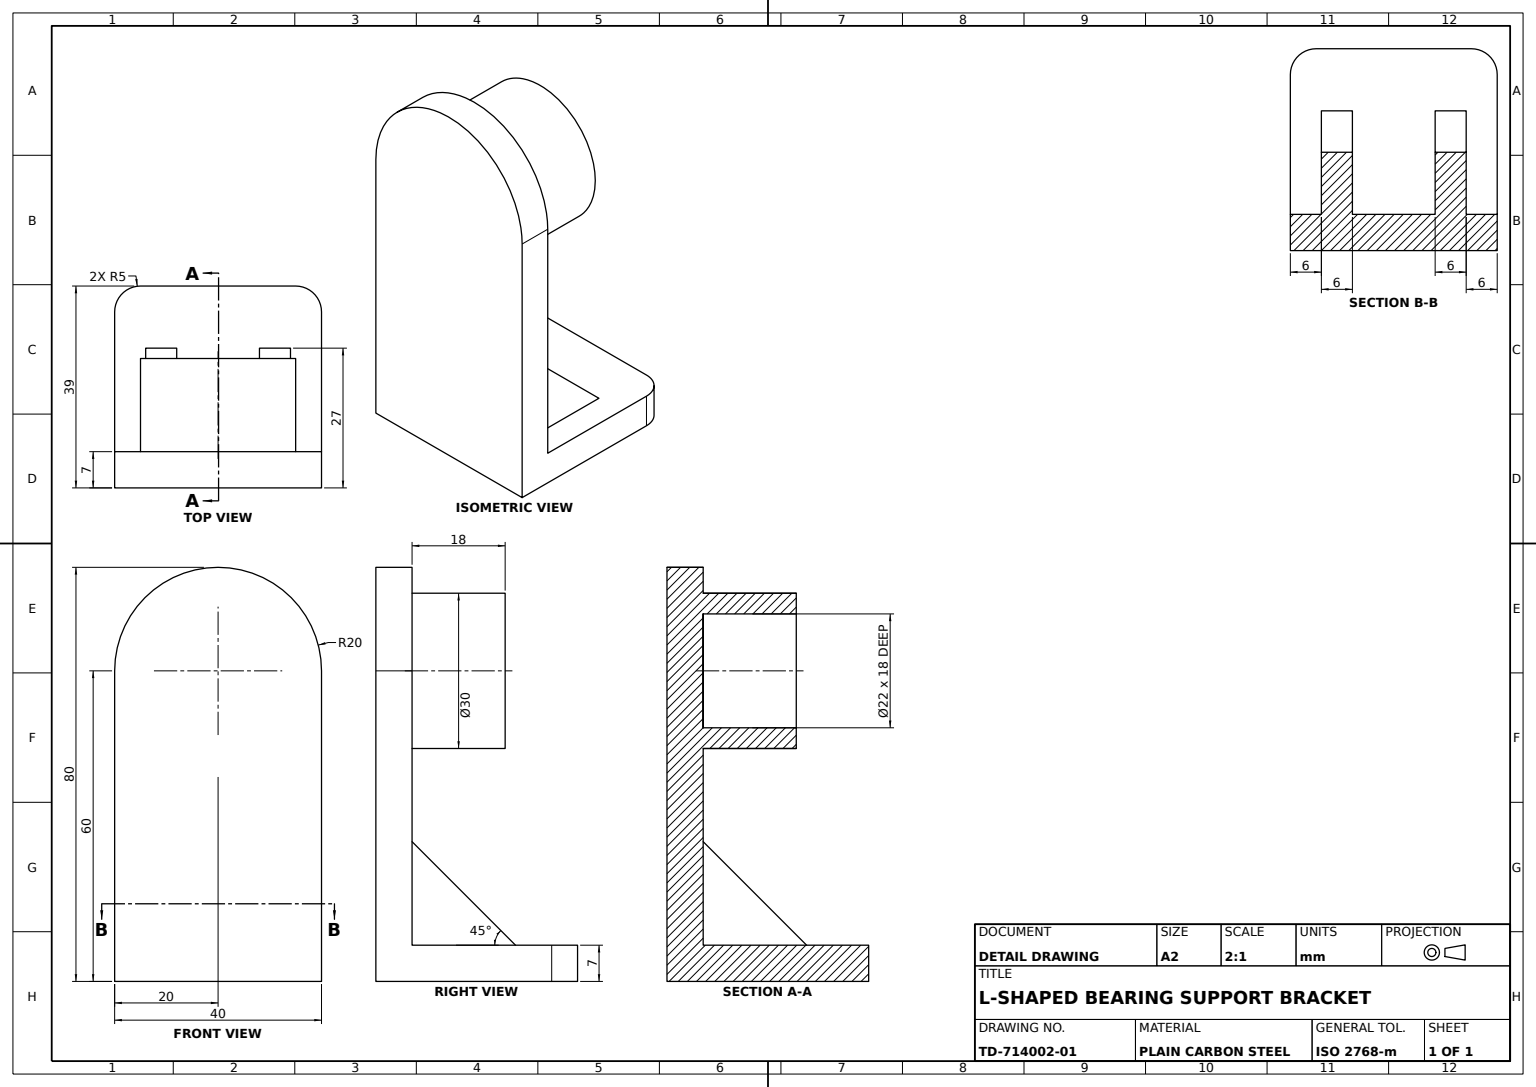
SolidWorks part; units mm, degrees
material "Plain Carbon Steel"
ref_plane "Front Plane" through (0, 0, 0) normal (0, 0, 1) x (1, 0, 0)
ref_plane "Top Plane" through (0, 0, 0) normal (0, 1, 0) x (1, 0, 0)
ref_plane "Right Plane" through (0, 0, 0) normal (1, 0, 0) x (0, 0, -1)
sketch "L Profile Sketch" plane through (0, 0, 0) normal (0, 0, 1) x (1, 0, 0)
  line L0 (0, 0) -> (34, 0)
  line L1 (34, 0) -> (34, 60)
  line L2 (34, 60) -> (27, 60)
  line L3 (0, 0) -> (0, 7)
  line L4 (0, 7) -> (27, 7)
  line L5 (27, 7) -> (27, 60)
  dimension "D1" = 27
  dimension "D2" = 34
  dimension "D3" = 60
extrude "L Bracket Base" add sketch "L Profile Sketch" along normal blind 40
sketch "Corner Block Sketch" plane through (0, 7, 0) normal (0, 1, 0) x (1, 0, 0)
  line L1 (0, -40) -> (0, 0) construction
  line L3 (-5, -5) -> (-5, -35)
  line L6 (27, 0) -> (0, 0)
  line L7 (0, 0) -> (0, -40)
  line L8 (0, -40) -> (27, -40)
  line L9 (27, -40) -> (27, 0)
  line L11 (0, 0) -> (0, -40)
  arc A0 (0, 0) -> (-5, -5) centre (0, -5) ccw
  arc A1 (-5, -35) -> (0, -40) centre (0, -35) ccw
  dimension "D1" = 10
  dimension "D2" = 10
  dimension "D4" = 5
  dimension "D3" = 0
extrude "Corner Block" add sketch "Corner Block Sketch" against normal blind 7
sketch "Upright Top Arc Sketch" plane through (27, 0, 0) normal (-1, 0, 0) x (0, 0, 1)
  line L0 (40, 60) -> (0, 60) construction
  line L1 (0, 60) -> (40, 60)
  arc A0 (40, 60) -> (0, 60) centre (20, 60) ccw
  dimension "D1" = 40
extrude "Upright Rounded Top" add sketch "Upright Top Arc Sketch" against normal blind 7
sketch "Hub Sketch Ø30" plane through (27, 0, 0) normal (-1, 0, 0) x (0, 0, 1)
  circle A0 centre (20, 60) radius 15
  dimension "D1" = 30
  dimension "D2" = 30
extrude "Hub Ø30" add sketch "Hub Sketch Ø30" along normal blind 18
sketch "Bore Sketch Ø22" plane through (9, 0, 0) normal (-1, 0, 0) x (0, 0, 1)
  circle A0 centre (20, 60) radius 11
  dimension "D1" = 22
  dimension "D2" = 22
extrude "Bore Ø22" cut sketch "Bore Sketch Ø22" against normal blind 18
sketch "Rib 1 Sketch" plane through (0, 0, 40) normal (0, 0, 1) x (1, 0, 0)
  line L0 (27, 7) -> (27, 27)
  line L1 (27, 60) -> (27, 7) construction
  line L2 (27, 7) -> (7, 7)
  line L3 (27, 7) -> (0, 7) construction
  line L4 (7, 7) -> (27, 27)
  line L5 (0, 7) -> (0, 0) construction
  dimension "D1" = 7
extrude "Rib 1" add sketch "Rib 1 Sketch" against normal blind 12
sketch "Rib 2 Sketch" plane through (0, 0, 0) normal (0, 0, -1) x (-1, 0, 0)
  line L0 (-27, 7) -> (-7, 7)
  line L1 (-7, 7) -> (-27, 27)
  line L2 (-27, 27) -> (-27, 7)
extrude "Rib 2" add sketch "Rib 2 Sketch" against normal blind 12
sketch "Triangular Cut 1 Sketch" plane through (0, 0, 0) normal (0, 0, -1) x (-1, 0, 0)
  line L0 (-27, 27) -> (-7, 7)
  line L1 (-7, 7) -> (-27, 7)
  line L2 (-27, 7) -> (-27, 27)
extrude "Triangular Cut 1" cut sketch "Triangular Cut 1 Sketch" against normal blind 6
sketch "Triangular Cut 2 Sketch" plane through (0, 0, 40) normal (0, 0, 1) x (1, 0, 0)
  line L0 (27, 27) -> (7, 7)
  line L1 (7, 7) -> (27, 7)
  line L2 (27, 7) -> (27, 27)
extrude "Triangular Cut 2" cut sketch "Triangular Cut 2 Sketch" against normal blind 6
